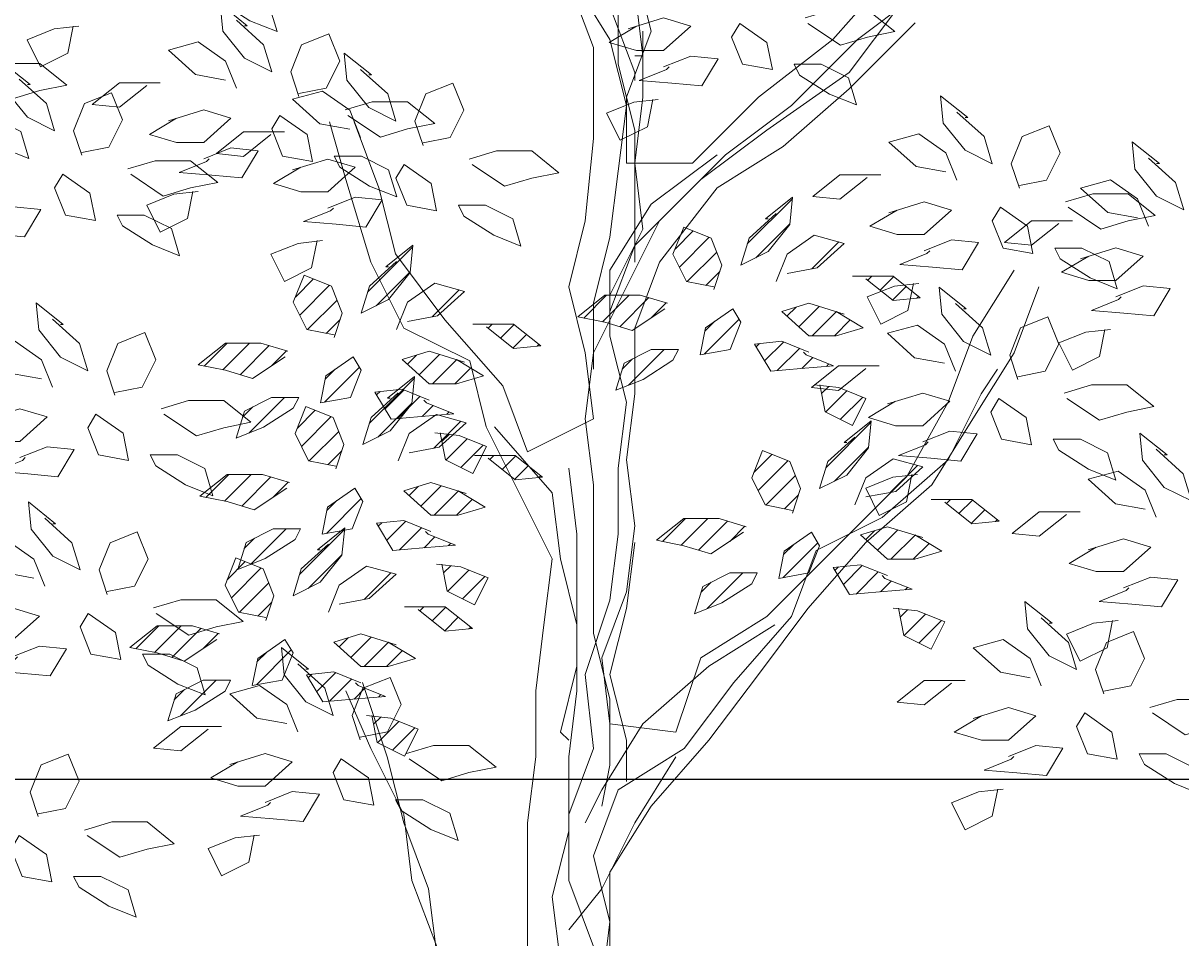
# Model space of a CAD drawing. Units: inches. Extents: x 1770 to 2988, y 1161 to 3221.
# Tile 40 of 44: x 2687 to 2745, y 2750 to 2796. Entities that reach past the tile are written whole.
import ezdxf

# ---------------------------------------------------------------- set-up
doc = ezdxf.new("R2010")
doc.units = ezdxf.units.IN
doc.layers.add('A-ANNO-DIMS', color=2, linetype='Continuous', lineweight=18)
doc.layers.add('trees1', color=250, linetype='Continuous', lineweight=13)
doc.styles.get("Standard").update_dxf_attribs({"font": 'arial.ttf'})
doc.dimstyles.get("Standard").update_dxf_attribs({"dimtxt": 0.18, "dimasz": 0.18, "dimexe": 0.18, "dimexo": 0.0625, "dimgap": 0.09, "dimtad": 0, "dimtih": 1, "dimtoh": 1, "dimdec": 4, "dimzin": 0, "dimdsep": 46, "dimtxsty": 'Standard', "dimcen": 0.09, "dimadec": 0, "dimazin": 0, "dimtfac": 1, "dimtdec": 4, "dimtofl": 0, "dimtmove": 0, "dimatfit": 3, "dimfxl": 1, "dimtolj": 1, "dimtzin": 0, "dimarcsym": 0})

# ---------------------------------------------------------------- blocks, each defined once
blk = doc.blocks.new('*X12')
at = {"color": 0}
for p, q in [((0.47641, -0.84941), (0.49451, -0.83131)), ((0.49114, -0.85236), (0.51219, -0.83131)), ((0.5049, -0.85628), (0.52785, -0.83333)), ((0.52956, -0.8493), (0.54145, -0.83741))]:
    blk.add_line(p, q, dxfattribs=at)
blk = doc.blocks.new('*X10')
at = {"color": 0}
for p, q in [((0.51178, -0.90243), (0.53998, -0.87423)), ((0.50681, -0.88973), (0.5149, -0.88163))]:
    blk.add_line(p, q, dxfattribs=at)
blk = doc.blocks.new('*X15')
at = {"color": 0}
for p, q in [((0.60562, -0.79091), (0.64126, -0.75528)), ((0.61243, -0.80179), (0.63929, -0.77492))]:
    blk.add_line(p, q, dxfattribs=at)
blk = doc.blocks.new('*X14')
at = {"color": 0}
blk.add_line((0.65666, -0.81059), (0.67788, -0.78936), dxfattribs=at)
blk = doc.blocks.new('*X6')
at = {"color": 0}
for p, q in [((0.61933, -0.88328), (0.63423, -0.86837)), ((0.61269, -0.87223), (0.61539, -0.86953)), ((0.62935, -0.89093), (0.64686, -0.87342)), ((0.64878, -0.88917), (0.65735, -0.88061)), ((0.66807, -0.88757), (0.66997, -0.88566))]:
    blk.add_line(p, q, dxfattribs=at)
blk = doc.blocks.new('*X8')
at = {"color": 0}
for p, q in [((0.63698, -0.84795), (0.64414, -0.84079)), ((0.64628, -0.85632), (0.66236, -0.84024)), ((0.65678, -0.8635), (0.67596, -0.84432)), ((0.67446, -0.8635), (0.68701, -0.85095))]:
    blk.add_line(p, q, dxfattribs=at)
blk = doc.blocks.new('*X9')
at = {"color": 0}
for p, q in [((0.70074, -0.81954), (0.70399, -0.81629)), ((0.71057, -0.82739), (0.7213, -0.81666)), ((0.72039, -0.83525), (0.73112, -0.82451)), ((0.73958, -0.83373), (0.74095, -0.83237))]:
    blk.add_line(p, q, dxfattribs=at)
blk = doc.blocks.new('*X7')
at = {"color": 0}
for p, q in [((0.66425, -0.90907), (0.66992, -0.90339)), ((0.66732, -0.92367), (0.68419, -0.9068)), ((0.67911, -0.92956), (0.69682, -0.91184))]:
    blk.add_line(p, q, dxfattribs=at)
blk = doc.blocks.new('*X13')
at = {"color": 0}
for p, q in [((0.54857, -0.79493), (0.56288, -0.78062)), ((0.55195, -0.80923), (0.57551, -0.78567)), ((0.55817, -0.82069), (0.58143, -0.79742)), ((0.5729, -0.82363), (0.58391, -0.81263))]:
    blk.add_line(p, q, dxfattribs=at)
blk = doc.blocks.new('*X11')
at = {"color": 0}
for p, q in [((0.57164, -0.87793), (0.59916, -0.85041)), ((0.57212, -0.85977), (0.57987, -0.85203))]:
    blk.add_line(p, q, dxfattribs=at)
blk = doc.blocks.new('tree342')
at = {"color": 0}
for p, q in [((-39.1, 1419.59), (-39.1, 1315.4)), ((-26.06, 1393.54), (-13.03, 1341.45)), ((130.32, 1334.94), (182.45, 1393.54)), ((-78.19, 1387.03), (-45.61, 1334.94)), ((-58.65, 1328.42), (-78.19, 1380.52)), ((-26.06, 1374.01), (-19.55, 1321.91)), ((202, 1374.01), (149.87, 1334.94)), ((-45.61, 1360.98), (-26.06, 1308.89)), ((182.45, 1360.98), (143.36, 1308.89)), ((195.49, 1347.96), (143.36, 1295.86)), ((-13.03, 1341.45), (-32.58, 1289.35)), ((-19.55, 1289.35), (-19.55, 1341.45)), ((-58.65, 1256.79), (-58.65, 1328.42)), ((-45.61, 1334.94), (-32.58, 1282.84)), ((71.68, 1289.35), (130.32, 1334.94)), ((149.87, 1334.94), (97.74, 1282.84)), ((-19.55, 1321.91), (-26.06, 1321.91)), ((-39.1, 1315.4), (-26.06, 1263.3)), ((-26.06, 1308.89), (-26.06, 1302.38)), ((143.36, 1308.89), (78.19, 1263.3)), ((143.36, 1295.86), (91.23, 1250.28)), ((-32.58, 1282.84), (-39.1, 1230.75)), ((-32.58, 1289.35), (-32.58, 1237.26)), ((-26.06, 1237.26), (-19.55, 1289.35)), ((19.55, 1237.26), (71.68, 1289.35)), ((97.74, 1282.84), (45.61, 1243.77)), ((-254.13, 1224.23), (-267.17, 1269.82)), ((-247.62, 1269.82), (-228.07, 1217.72)), ((-26.06, 1263.3), (-26.06, 1159.11)), ((78.19, 1263.3), (26.06, 1224.23)), ((-65.16, 1191.67), (-58.65, 1256.79)), ((45.61, 1243.77), (-6.52, 1191.67)), ((91.23, 1250.28), (39.1, 1217.72)), ((-32.58, 1237.26), (19.55, 1237.26)), ((-19.55, 1185.16), (-26.06, 1237.26)), ((-39.1, 1230.75), (-45.61, 1178.65)), ((-234.58, 1159.11), (-254.13, 1224.23)), ((-228.07, 1217.72), (-215.04, 1165.63)), ((26.06, 1224.23), (-26.06, 1172.14)), ((39.1, 1217.72), (-6.52, 1159.11)), ((-78.19, 1139.58), (-65.16, 1191.67)), ((-6.52, 1191.67), (-58.65, 1087.48)), ((-45.61, 1133.07), (-19.55, 1185.16)), ((-45.61, 1178.65), (-58.65, 1126.56)), ((-26.06, 1172.14), (-45.61, 1120.04)), ((-215.04, 1165.63), (-175.94, 1113.53)), ((-208.52, 1107.02), (-234.58, 1159.11)), ((-6.52, 1159.11), (-26.06, 1107.02)), ((241.1, 1100.51), (273.68, 1152.6)), ((-65.16, 1087.48), (-78.19, 1139.58)), ((-58.65, 1126.56), (-58.65, 1074.46)), ((-45.61, 1113.53), (-45.61, 1133.07)), ((-45.61, 1120.04), (-45.61, 1113.53)), ((-156.39, 1080.97), (-208.52, 1107.02)), ((-175.94, 1113.53), (-130.32, 1061.44)), ((-26.06, 1107.02), (-26.06, 1054.92)), ((221.55, 1048.41), (241.1, 1100.51)), ((-143.36, 1028.88), (-156.39, 1080.97)), ((-58.65, 1087.48), (-65.16, 1035.39)), ((-58.65, 1035.39), (-65.16, 1087.48)), ((-130.32, 1061.44), (-110.78, 1009.34)), ((-26.06, 1054.92), (-32.58, 1002.83)), ((188.97, 989.81), (221.55, 1048.41)), ((-110.78, 1009.34), (-58.65, 1035.39)), ((-65.16, 1035.39), (-58.65, 983.29)), ((-91.23, 924.69), (-143.36, 1028.88)), ((-32.58, 1002.83), (-26.06, 950.73)), ((-78.19, 996.32), (-71.68, 944.22)), ((78.19, 879.1), (188.97, 989.81)), ((-58.65, 983.29), (-58.65, 866.08)), ((-71.68, 944.22), (-71.68, 840.03)), ((-26.06, 950.73), (-32.58, 898.64)), ((-26.06, 937.71), (-32.58, 885.62)), ((-97.74, 872.59), (-91.23, 924.69)), ((-32.58, 898.64), (-52.13, 846.54)), ((-32.58, 885.62), (-45.61, 833.52)), ((26.06, 846.54), (78.19, 879.1)), ((-104.26, 820.5), (-97.74, 872.59)), ((84.71, 872.59), (32.58, 840.03)), ((-58.65, 866.08), (-45.61, 813.98)), ((-52.13, 846.54), (-45.61, 794.45)), ((6.52, 787.94), (26.06, 846.54)), ((-71.68, 840.03), (-84.71, 787.94)), ((-45.61, 833.52), (-32.58, 781.43)), ((32.58, 840.03), (-19.55, 794.45)), ((-241.1, 827.01), (-221.55, 768.4)), ((-104.26, 768.4), (-104.26, 820.5)), ((-45.61, 813.98), (-45.61, 761.89)), ((-84.71, 787.94), (-78.19, 781.43)), ((-19.55, 794.45), (-52.13, 742.35)), ((-45.61, 794.45), (6.52, 787.94)), ((-32.58, 781.43), (-32.58, 748.87)), ((-221.55, 768.4), (-208.52, 716.31)), ((-110.78, 716.31), (-104.26, 768.4)), ((6.52, 768.4), (-26.06, 716.31)), ((-45.61, 761.89), (-52.13, 729.33)), ((-52.13, 742.35), (-65.16, 716.31)), ((-208.52, 716.31), (-188.97, 664.21)), ((-110.78, 612.12), (-110.78, 716.31)), ((-26.06, 716.31), (-52.13, 664.21)), ((-188.97, 664.21), (-182.45, 612.12)), ((-52.13, 664.21), (-78.19, 631.65))]:
    blk.add_line(p, q, dxfattribs=at)
for points in [[(-336.45, 1373.29), (-314.97, 1362.56), (-308.53, 1341.1), (-330, 1349.68), (-353.63, 1364.71), (-357.92, 1373.29)], [(78.39, 1332.52), (82.69, 1311.06), (59.07, 1315.35), (50.48, 1336.81), (56.92, 1347.54)], [(121.34, 1315.35), (142.82, 1304.62), (149.26, 1283.16), (127.79, 1291.74), (104.16, 1306.77), (99.87, 1315.35)], [(-532.55, 1273), (-511.08, 1262.27), (-504.64, 1240.81), (-526.11, 1249.39), (-549.73, 1264.41), (-554.03, 1273)], [(-284.88, 1259.91), (-280.59, 1238.45), (-304.21, 1242.74), (-312.8, 1264.2), (-306.36, 1274.93)], [(-241.93, 1242.74), (-220.46, 1232.01), (-214.02, 1210.55), (-235.49, 1219.14), (-259.11, 1234.16), (-263.41, 1242.74)], [(-186.8, 1221.09), (-182.51, 1199.63), (-206.13, 1203.92), (-214.72, 1225.38), (-208.28, 1236.11)], [(-456.43, 1213.39), (-452.14, 1191.93), (-475.76, 1196.22), (-484.35, 1217.69), (-477.91, 1228.42)], [(-143.85, 1203.92), (-122.38, 1193.19), (-115.94, 1171.73), (-137.41, 1180.32), (-161.03, 1195.34), (-165.33, 1203.92)], [(284.25, 1187.31), (288.54, 1165.85), (264.92, 1170.14), (256.33, 1191.6), (262.78, 1202.33)], [(-413.48, 1196.22), (-392.01, 1185.49), (-385.57, 1164.03), (-407.04, 1172.62), (-430.66, 1187.64), (-434.96, 1196.22)], [(327.2, 1170.14), (348.67, 1159.41), (355.12, 1137.95), (333.64, 1146.53), (310.02, 1161.55), (305.72, 1170.14)], [(29.91, 1107.26), (25.62, 1085.8), (49.24, 1090.09), (57.83, 1111.55), (51.39, 1122.28)], [(-13.04, 1090.09), (-34.51, 1079.36), (-40.95, 1057.9), (-19.48, 1066.48), (4.14, 1081.5), (8.44, 1090.09)], [(-269.97, 1069.36), (-274.26, 1047.9), (-250.64, 1052.19), (-242.05, 1073.65), (-248.49, 1084.38)], [(-312.92, 1052.19), (-334.39, 1041.46), (-340.83, 1020), (-319.36, 1028.59), (-295.74, 1043.61), (-291.44, 1052.19)], [(283.12, 1036.33), (287.41, 1014.87), (263.79, 1019.16), (255.2, 1040.62), (261.64, 1051.35)], [(-430.19, 1023.94), (-425.9, 1002.48), (-449.52, 1006.78), (-458.11, 1028.24), (-451.67, 1038.97)], [(326.07, 1019.16), (347.54, 1008.43), (353.98, 986.97), (332.51, 995.55), (308.89, 1010.58), (304.59, 1019.16)], [(-387.24, 1006.78), (-365.77, 996.05), (-359.33, 974.59), (-380.8, 983.17), (-404.42, 998.19), (-408.72, 1006.78)], [(-268.62, 965.65), (-272.92, 944.19), (-249.3, 948.48), (-240.71, 969.94), (-247.15, 980.67)], [(-311.57, 948.48), (-333.05, 937.75), (-339.49, 916.29), (-318.02, 924.87), (-294.39, 939.9), (-290.1, 948.48)], [(92.1, 930.79), (87.81, 909.33), (111.43, 913.62), (120.02, 935.08), (113.58, 945.81)], [(49.15, 913.62), (27.68, 902.89), (21.24, 881.43), (42.71, 890.01), (66.33, 905.04), (70.63, 913.62)], [(-436.25, 866.63), (-431.95, 845.17), (-455.57, 849.46), (-464.16, 870.92), (-457.72, 881.65)], [(-323.89, 846.1), (-328.19, 824.64), (-304.57, 828.94), (-295.98, 850.4), (-302.42, 861.13)], [(-393.3, 849.46), (-371.82, 838.73), (-365.38, 817.27), (-386.85, 825.86), (-410.48, 840.88), (-414.77, 849.46)], [(-366.84, 828.94), (-388.32, 818.21), (-394.76, 796.75), (-373.29, 805.33), (-349.66, 820.35), (-345.37, 828.94)], [(350.85, 787.97), (355.15, 766.51), (331.52, 770.81), (322.93, 792.27), (329.38, 803)], [(393.8, 770.81), (415.27, 760.08), (421.72, 738.62), (400.24, 747.2), (376.62, 762.22), (372.32, 770.81)], [(-236.44, 751.67), (-232.15, 730.21), (-255.77, 734.5), (-264.36, 755.96), (-257.92, 766.69)], [(-193.5, 734.5), (-172.02, 723.77), (-165.58, 702.31), (-187.05, 710.9), (-210.67, 725.92), (-214.97, 734.5)], [(-490.74, 691.17), (-486.44, 669.71), (-510.06, 674), (-518.65, 695.46), (-512.21, 706.19)], [(-447.79, 674), (-426.31, 663.27), (-419.87, 641.81), (-441.35, 650.39), (-464.97, 665.41), (-469.26, 674)]]:
    blk.add_lwpolyline(points, close=True, dxfattribs=at)
for points in [[(-340.71, 1350.05), (-319.24, 1330.73), (-312.8, 1309.27), (-334.27, 1320), (-351.45, 1341.46), (-353.6, 1362.92), (-332.12, 1345.75), (-334.27, 1345.75)], [(110.61, 1347.54), (136.38, 1330.37), (157.85, 1336.81), (179.32, 1341.1), (157.85, 1358.27), (129.93, 1358.27), (108.46, 1351.83)], [(-469.59, 1345.39), (-473.88, 1323.93), (-495.36, 1313.2), (-506.09, 1334.66), (-484.62, 1343.25), (-465.29, 1345.39)], [(-31.13, 1343.25), (-3.21, 1351.83), (18.27, 1345.39), (-3.21, 1326.08), (-24.68, 1326.08), (-46.16, 1332.52), (-24.68, 1345.39)], [(-291.32, 1292.1), (-269.85, 1296.39), (-259.11, 1317.86), (-267.7, 1339.32), (-289.18, 1330.73), (-297.77, 1309.27), (-291.32, 1289.96)], [(-340.71, 1296.39), (-349.3, 1317.86), (-370.78, 1332.88), (-394.4, 1326.44), (-372.93, 1307.13), (-349.3, 1302.83)], [(-242.64, 1311.22), (-221.16, 1291.91), (-214.72, 1270.45), (-236.19, 1281.18), (-253.37, 1302.64), (-255.52, 1324.1), (-234.05, 1306.93), (-236.19, 1306.93)], [(-3.21, 1313.2), (18.27, 1321.79), (39.74, 1319.64), (26.86, 1298.18), (3.23, 1300.33), (-22.54, 1302.47), (-1.06, 1311.06), (1.09, 1313.2)], [(-543.29, 1305.19), (-517.52, 1288.02), (-496.05, 1294.46), (-474.57, 1298.75), (-496.05, 1315.92), (-523.96, 1315.92), (-545.44, 1309.48)], [(-512.26, 1303.53), (-490.79, 1284.21), (-484.35, 1262.75), (-505.82, 1273.48), (-523, 1294.94), (-525.15, 1316.4), (-503.67, 1299.23), (-505.82, 1299.23)], [(-411.58, 1298.54), (-433.05, 1281.37), (-454.53, 1283.52), (-433.05, 1300.69), (-400.84, 1300.69)], [(-193.25, 1253.28), (-171.77, 1257.57), (-161.03, 1279.03), (-169.62, 1300.49), (-191.1, 1291.91), (-199.69, 1270.45), (-193.25, 1251.14)], [(-462.87, 1245.58), (-441.4, 1249.88), (-430.66, 1271.34), (-439.25, 1292.8), (-460.73, 1284.21), (-469.32, 1262.75), (-462.87, 1243.44)], [(-242.64, 1257.57), (-251.23, 1279.03), (-272.7, 1294.06), (-296.32, 1287.62), (-274.85, 1268.3), (-251.23, 1264.01)], [(228.42, 1277.44), (249.89, 1258.13), (256.33, 1236.67), (234.86, 1247.4), (217.68, 1268.86), (215.53, 1290.32), (237.01, 1273.15), (234.86, 1273.15)], [(-252.67, 1274.93), (-226.9, 1257.77), (-205.43, 1264.2), (-183.95, 1268.5), (-205.43, 1285.66), (-233.34, 1285.66), (-254.82, 1279.23)], [(-11.8, 1287.45), (-16.09, 1265.99), (-37.57, 1255.26), (-48.31, 1276.72), (-26.83, 1285.31), (-7.5, 1287.45)], [(-394.4, 1270.64), (-366.48, 1279.23), (-345.01, 1272.79), (-366.48, 1253.47), (-387.96, 1253.47), (-409.43, 1259.91), (-387.96, 1272.79)], [(277.81, 1219.5), (299.28, 1223.79), (310.02, 1245.25), (301.43, 1266.71), (279.95, 1258.13), (271.37, 1236.67), (277.81, 1217.35)], [(-313.5, 1259.72), (-334.98, 1242.55), (-356.45, 1244.7), (-334.98, 1261.87), (-302.77, 1261.87)], [(228.42, 1223.79), (219.83, 1245.25), (198.35, 1260.27), (174.73, 1253.83), (196.2, 1234.52), (219.83, 1230.23)], [(379.78, 1241.14), (401.26, 1221.82), (407.7, 1200.36), (386.22, 1211.09), (369.04, 1232.55), (366.9, 1254.01), (388.37, 1236.84), (386.22, 1236.84)], [(-366.48, 1240.6), (-345.01, 1249.18), (-323.53, 1247.04), (-336.42, 1225.58), (-360.04, 1227.72), (-385.81, 1229.87), (-364.34, 1238.45), (-362.19, 1240.6)], [(-154.59, 1236.11), (-128.82, 1218.95), (-107.35, 1225.38), (-85.87, 1229.68), (-107.35, 1246.84), (-135.27, 1246.84), (-156.74, 1240.41)], [(39.1, 1243.77), (-13.03, 1204.7), (-45.61, 1152.6), (-45.61, 1100.51), (-32.58, 1048.41), (-39.1, 996.32), (-39.1, 944.22), (-45.61, 892.13), (-65.16, 833.52), (-58.65, 774.91), (-78.19, 722.82), (-78.19, 670.72), (-58.65, 618.63), (-65.16, 566.53), (-65.16, 514.44), (-78.19, 462.34), (-84.71, 410.25), (-84.71, 306.06), (-78.19, 247.45), (-71.68, 195.36), (-78.19, 143.26), (-71.68, 91.17), (-65.16, 32.56), (-65.16, 0)], [(-424.22, 1228.42), (-398.45, 1211.25), (-376.98, 1217.69), (-355.5, 1221.98), (-376.98, 1239.15), (-404.89, 1239.15), (-426.37, 1232.71)], [(-296.32, 1231.82), (-268.41, 1240.41), (-246.93, 1233.97), (-268.41, 1214.65), (-289.88, 1214.65), (-311.36, 1221.09), (-289.88, 1233.97)], [(157.55, 1225.94), (136.08, 1208.77), (114.6, 1210.91), (136.08, 1228.08), (168.29, 1228.08)], [(379.78, 1187.49), (371.19, 1208.95), (349.72, 1223.97), (326.09, 1217.53), (347.57, 1198.22), (371.19, 1193.92)], [(-375.07, 1214.85), (-379.37, 1193.39), (-400.84, 1182.66), (-411.58, 1204.12), (-390.11, 1212.7), (-370.78, 1214.85)], [(-268.41, 1201.78), (-246.93, 1210.36), (-225.46, 1208.22), (-238.34, 1186.76), (-261.96, 1188.9), (-287.73, 1191.05), (-266.26, 1199.63), (-264.11, 1201.78)], [(85.75, 1197.39), (64.27, 1178.07), (57.83, 1156.61), (79.3, 1167.34), (96.48, 1188.8), (98.63, 1210.26), (77.16, 1193.1), (79.3, 1193.1)], [(316.46, 1202.33), (342.23, 1185.16), (363.71, 1191.6), (385.18, 1195.89), (363.71, 1213.06), (335.79, 1213.06), (314.31, 1206.62)], [(-538.03, 1194.08), (-516.56, 1202.66), (-495.09, 1200.52), (-507.97, 1179.06), (-531.59, 1181.2), (-557.36, 1183.35), (-535.89, 1191.93), (-533.74, 1194.08)], [(174.73, 1198.04), (202.65, 1206.62), (224.12, 1200.18), (202.65, 1180.87), (181.17, 1180.87), (159.7, 1187.31), (181.17, 1200.18)], [(308.92, 1189.63), (287.44, 1172.46), (265.97, 1174.61), (287.44, 1191.78), (319.65, 1191.78)], [(36.36, 1139.45), (14.88, 1143.74), (4.14, 1165.2), (12.73, 1186.66), (34.21, 1178.07), (42.8, 1156.61), (36.36, 1137.3)], [(85.75, 1143.74), (94.34, 1165.2), (115.81, 1180.22), (139.43, 1173.78), (117.96, 1154.47), (94.34, 1150.18)], [(-277, 1176.03), (-281.29, 1154.57), (-302.77, 1143.84), (-313.5, 1165.3), (-292.03, 1173.88), (-272.7, 1176.03)], [(-214.14, 1159.49), (-235.61, 1140.18), (-242.05, 1118.72), (-220.58, 1129.45), (-203.4, 1150.91), (-201.25, 1172.37), (-222.72, 1155.2), (-220.58, 1155.2)], [(202.65, 1167.99), (224.12, 1176.58), (245.6, 1174.43), (232.71, 1152.97), (209.09, 1155.12), (183.32, 1157.26), (204.79, 1165.85), (206.94, 1167.99)], [(326.09, 1161.73), (354.01, 1170.32), (375.49, 1163.88), (354.01, 1144.57), (332.54, 1144.57), (311.06, 1151), (332.54, 1163.88)], [(-263.53, 1101.55), (-285, 1105.84), (-295.74, 1127.3), (-287.15, 1148.76), (-265.67, 1140.18), (-257.08, 1118.72), (-263.53, 1099.4)], [(156.61, 1145.88), (178.09, 1128.72), (199.56, 1130.86), (178.09, 1148.03), (145.88, 1148.03)], [(-214.14, 1105.84), (-205.55, 1127.3), (-184.07, 1142.32), (-160.45, 1135.89), (-181.92, 1116.57), (-205.55, 1112.28)], [(293.23, 1139.58), (273.68, 1087.48), (241.1, 1035.39), (208.52, 983.29), (156.39, 937.71), (110.78, 885.62), (71.68, 833.52), (32.58, 781.43), (-13.03, 729.33), (-45.61, 677.24), (-45.61, 566.53), (-39.1, 507.93), (-45.61, 455.83), (-45.61, 403.74), (-39.1, 345.13), (-58.65, 293.03), (-58.65, 188.84), (-65.16, 136.75), (-58.65, 84.65), (-52.13, 32.56), (-45.61, 13.02)], [(194.06, 1142.24), (189.76, 1120.78), (168.29, 1110.05), (157.55, 1131.51), (179.03, 1140.09), (198.35, 1142.24)], [(227.28, 1126.46), (248.76, 1107.15), (255.2, 1085.69), (233.73, 1096.42), (216.55, 1117.88), (214.4, 1139.34), (235.87, 1122.17), (233.73, 1122.17)], [(354.01, 1131.69), (375.49, 1140.27), (396.96, 1138.13), (384.08, 1116.67), (360.45, 1118.81), (334.68, 1120.96), (356.16, 1129.54), (358.31, 1131.69)], [(-486.02, 1114.08), (-464.55, 1094.76), (-458.11, 1073.3), (-479.58, 1084.03), (-496.76, 1105.49), (-498.91, 1126.95), (-477.43, 1109.78), (-479.58, 1109.78)], [(-2.3, 1122.28), (-28.07, 1105.11), (-49.54, 1111.55), (-71.02, 1115.84), (-49.54, 1133.01), (-21.63, 1133.01), (-0.15, 1126.57)], [(139.43, 1117.99), (111.52, 1126.57), (90.04, 1120.13), (111.52, 1100.82), (132.99, 1100.82), (154.46, 1107.26), (132.99, 1120.13)], [(276.68, 1068.52), (298.15, 1072.81), (308.89, 1094.27), (300.3, 1115.73), (278.82, 1107.15), (270.23, 1085.69), (276.68, 1066.37)], [(-143.27, 1107.99), (-121.8, 1090.82), (-100.32, 1092.97), (-121.8, 1110.13), (-154.01, 1110.13)], [(227.28, 1072.81), (218.69, 1094.27), (197.22, 1109.29), (173.6, 1102.85), (195.07, 1083.54), (218.69, 1079.25)], [(-436.63, 1056.13), (-415.16, 1060.43), (-404.42, 1081.89), (-413.01, 1103.35), (-434.49, 1094.76), (-443.08, 1073.3), (-436.63, 1053.99)], [(345.42, 1105.94), (341.13, 1084.48), (319.65, 1073.75), (308.92, 1095.21), (330.39, 1103.79), (349.72, 1105.94)], [(-486.02, 1060.43), (-494.61, 1081.89), (-516.09, 1096.91), (-539.71, 1090.47), (-518.24, 1071.16), (-494.61, 1066.86)], [(-302.18, 1084.38), (-327.95, 1067.21), (-349.42, 1073.65), (-370.9, 1077.94), (-349.42, 1095.11), (-321.51, 1095.11), (-300.03, 1088.67)], [(-160.45, 1080.09), (-188.37, 1088.67), (-209.84, 1082.24), (-188.37, 1062.92), (-166.89, 1062.92), (-145.42, 1069.36), (-166.89, 1082.24)], [(111.52, 1087.94), (90.04, 1096.53), (68.57, 1094.38), (81.45, 1072.92), (105.07, 1075.07), (130.84, 1077.21), (109.37, 1085.8), (107.22, 1087.94)], [(-65.16, 6.51), (-91.23, 58.61), (-84.71, 110.7), (-84.71, 162.8), (-78.19, 214.89), (-58.65, 266.99), (-52.13, 319.08), (-65.16, 371.18), (-52.13, 429.78), (-52.13, 481.88), (-45.61, 533.97), (-52.13, 586.07), (-45.61, 638.16), (-58.65, 690.26), (-39.1, 742.35), (13.03, 774.91), (52.13, 827.01), (97.74, 879.1), (117.29, 931.2), (169.42, 957.25), (221.55, 1002.83), (247.62, 1054.92), (260.65, 1074.46)], [(156.42, 1074.96), (134.94, 1057.79), (113.47, 1059.93), (134.94, 1077.1), (167.16, 1077.1)], [(-212.79, 1055.78), (-234.27, 1036.47), (-240.71, 1015.01), (-219.23, 1025.74), (-202.05, 1047.2), (-199.91, 1068.66), (-221.38, 1051.49), (-219.23, 1051.49)], [(120.11, 1062.19), (124.4, 1040.73), (145.88, 1030), (156.61, 1051.46), (135.14, 1060.04), (115.81, 1062.19)], [(315.33, 1051.35), (341.1, 1034.18), (362.57, 1040.62), (384.05, 1044.91), (362.57, 1062.08), (334.66, 1062.08), (313.18, 1055.64)], [(-188.37, 1050.05), (-209.84, 1058.63), (-231.31, 1056.48), (-218.43, 1035.02), (-194.81, 1037.17), (-169.04, 1039.32), (-190.51, 1047.9), (-192.66, 1050.05)], [(173.6, 1047.06), (201.52, 1055.64), (222.99, 1049.2), (201.52, 1029.89), (180.04, 1029.89), (158.57, 1036.33), (180.04, 1049.2)], [(-539.71, 1034.67), (-511.79, 1043.26), (-490.32, 1036.82), (-511.79, 1017.51), (-533.27, 1017.51), (-554.74, 1023.94), (-533.27, 1036.82)], [(-397.98, 1038.97), (-372.21, 1021.8), (-350.74, 1028.24), (-329.26, 1032.53), (-350.74, 1049.7), (-378.65, 1049.7), (-400.13, 1043.26)], [(-262.18, 997.84), (-283.66, 1002.13), (-294.39, 1023.59), (-285.8, 1045.05), (-264.33, 1036.47), (-255.74, 1015.01), (-262.18, 995.69)], [(-212.79, 1002.13), (-204.2, 1023.59), (-182.73, 1038.61), (-159.11, 1032.17), (-180.58, 1012.86), (-204.2, 1008.57)], [(147.94, 1020.92), (126.46, 1001.61), (120.02, 980.15), (141.49, 990.88), (158.67, 1012.34), (160.82, 1033.8), (139.35, 1016.63), (141.49, 1016.63)], [(-179.78, 1024.29), (-175.48, 1002.83), (-154.01, 992.1), (-143.27, 1013.56), (-164.74, 1022.15), (-184.07, 1024.29)], [(-136.84, 1028.88), (-91.23, 976.78), (-84.71, 924.69), (-71.68, 872.59), (-71.68, 820.5), (-78.19, 768.4), (-78.19, 709.79), (-91.23, 657.7), (-84.71, 605.6), (-78.19, 553.51), (-84.71, 501.41), (-97.74, 449.32), (-97.74, 410.25)], [(201.52, 1017.01), (222.99, 1025.6), (244.46, 1023.45), (231.58, 1001.99), (207.96, 1004.14), (182.19, 1006.28), (203.66, 1014.87), (205.81, 1017.01)], [(385.84, 1011.22), (407.31, 991.9), (413.75, 970.44), (392.28, 981.17), (375.1, 1002.63), (372.95, 1024.09), (394.43, 1006.93), (392.28, 1006.93)], [(-511.79, 1004.63), (-490.32, 1013.21), (-468.84, 1011.07), (-481.73, 989.61), (-505.35, 991.75), (-531.12, 993.9), (-509.65, 1002.48), (-507.5, 1004.63)], [(-141.93, 1004.28), (-120.45, 987.11), (-98.98, 989.25), (-120.45, 1006.42), (-152.66, 1006.42)], [(98.54, 962.98), (77.07, 967.27), (66.33, 988.73), (74.92, 1010.19), (96.4, 1001.61), (104.99, 980.15), (98.54, 960.83)], [(147.94, 967.27), (156.53, 988.73), (178, 1003.75), (201.62, 997.31), (180.15, 978), (156.53, 973.71)], [(-300.84, 980.67), (-326.61, 963.5), (-348.08, 969.94), (-369.55, 974.23), (-348.08, 991.4), (-320.16, 991.4), (-298.69, 984.96)], [(192.93, 991.26), (188.63, 969.8), (167.16, 959.07), (156.42, 980.53), (177.89, 989.12), (197.22, 991.26)], [(385.84, 957.57), (377.25, 979.03), (355.77, 994.05), (332.15, 987.61), (353.62, 968.3), (377.25, 964.01)], [(-159.11, 976.38), (-187.02, 984.96), (-208.5, 978.52), (-187.02, 959.21), (-165.55, 959.21), (-144.07, 965.65), (-165.55, 978.52)], [(-492.08, 956.76), (-470.6, 937.45), (-464.16, 915.99), (-485.64, 926.72), (-502.82, 948.18), (-504.96, 969.64), (-483.49, 952.47), (-485.64, 952.47)], [(218.8, 969.42), (240.28, 952.25), (261.75, 954.39), (240.28, 971.56), (208.06, 971.56)], [(314.97, 959.71), (293.5, 942.54), (272.02, 944.69), (293.5, 961.86), (325.71, 961.86)], [(-187.02, 946.33), (-208.5, 954.92), (-229.97, 952.77), (-217.09, 931.31), (-193.46, 933.46), (-167.69, 935.6), (-189.17, 944.19), (-191.32, 946.33)], [(59.89, 945.81), (34.12, 928.64), (12.65, 935.08), (-8.83, 939.37), (12.65, 956.54), (40.56, 956.54), (62.04, 950.1)], [(-442.69, 898.82), (-421.21, 903.11), (-410.48, 924.57), (-419.07, 946.03), (-440.54, 937.45), (-449.13, 915.99), (-442.69, 896.67)], [(-268.06, 936.24), (-289.54, 916.92), (-295.98, 895.46), (-274.5, 906.19), (-257.32, 927.65), (-255.18, 949.11), (-276.65, 931.94), (-274.5, 931.94)], [(201.62, 941.52), (173.71, 950.1), (152.23, 943.66), (173.71, 924.35), (195.18, 924.35), (216.65, 930.79), (195.18, 943.66)], [(-492.08, 903.11), (-500.67, 924.57), (-522.14, 939.59), (-545.77, 933.16), (-524.29, 913.84), (-500.67, 909.55)], [(332.15, 931.81), (360.07, 940.4), (381.54, 933.96), (360.07, 914.65), (338.59, 914.65), (317.12, 921.08), (338.59, 933.96)], [(-317.45, 878.29), (-338.93, 882.59), (-349.66, 904.05), (-341.07, 925.51), (-319.6, 916.92), (-311.01, 895.46), (-317.45, 876.15)], [(-268.06, 882.59), (-259.47, 904.05), (-238, 919.07), (-214.37, 912.63), (-235.85, 893.32), (-259.47, 889.02)], [(-178.43, 920.58), (-174.14, 899.12), (-152.66, 888.39), (-141.93, 909.85), (-163.4, 918.44), (-182.73, 920.58)], [(173.71, 911.47), (152.23, 920.06), (130.76, 917.91), (143.64, 896.45), (167.26, 898.6), (193.03, 900.74), (171.56, 909.33), (169.41, 911.47)], [(360.07, 901.77), (381.54, 910.35), (403.01, 908.21), (390.13, 886.75), (366.51, 888.89), (340.74, 891.04), (362.21, 899.62), (364.36, 901.77)], [(-404.03, 881.65), (-378.26, 864.48), (-356.79, 870.92), (-335.32, 875.21), (-356.79, 892.38), (-384.71, 892.38), (-406.18, 885.94)], [(295.02, 878.11), (316.49, 858.79), (322.93, 837.33), (301.46, 848.06), (284.28, 869.52), (282.13, 890.98), (303.61, 873.81), (301.46, 873.81)], [(-545.77, 877.36), (-517.85, 885.94), (-496.37, 879.51), (-517.85, 860.19), (-539.32, 860.19), (-560.8, 866.63), (-539.32, 879.51)], [(-197.2, 884.73), (-175.72, 867.56), (-154.25, 869.71), (-175.72, 886.88), (-207.93, 886.88)], [(182.29, 885.72), (186.59, 864.26), (208.06, 853.53), (218.8, 874.99), (197.33, 883.58), (178, 885.72)], [(-356.11, 861.13), (-381.88, 843.96), (-403.35, 850.4), (-424.82, 854.69), (-403.35, 871.86), (-375.43, 871.86), (-353.96, 865.42)], [(351.48, 876.02), (347.18, 854.56), (325.71, 843.83), (314.97, 865.29), (336.44, 873.87), (355.77, 876.02)], [(-214.37, 856.83), (-242.29, 865.42), (-263.77, 858.98), (-242.29, 839.67), (-220.82, 839.67), (-199.34, 846.1), (-220.82, 858.98)], [(295.02, 824.46), (286.43, 845.92), (264.95, 860.94), (241.33, 854.5), (262.8, 835.19), (286.43, 830.89)], [(344.41, 820.16), (365.88, 824.46), (376.62, 845.92), (368.03, 867.38), (346.56, 858.79), (337.97, 837.33), (344.41, 818.02)], [(-517.85, 847.32), (-496.37, 855.9), (-474.9, 853.75), (-487.78, 832.29), (-511.41, 834.44), (-537.18, 836.59), (-515.7, 845.17), (-513.55, 847.32)], [(-292.28, 841.8), (-270.8, 822.49), (-264.36, 801.03), (-285.84, 811.76), (-303.02, 833.22), (-305.16, 854.68), (-283.69, 837.51), (-285.84, 837.51)], [(-242.29, 826.79), (-263.77, 835.37), (-285.24, 833.23), (-272.36, 811.77), (-248.73, 813.91), (-222.96, 816.06), (-244.44, 824.64), (-246.59, 826.79)], [(-292.28, 788.15), (-300.87, 809.61), (-322.34, 824.64), (-345.96, 818.2), (-324.49, 798.88), (-300.87, 794.59)], [(-242.89, 783.86), (-221.41, 788.15), (-210.67, 809.61), (-219.26, 831.07), (-240.74, 822.49), (-249.33, 801.03), (-242.89, 781.72)], [(224.15, 826.6), (202.68, 809.43), (181.2, 811.58), (202.68, 828.75), (234.89, 828.75)], [(-162.91, 26.05), (-149.87, 78.14), (-143.36, 130.24), (-136.84, 188.84), (-130.32, 240.94), (-123.81, 293.03), (-110.78, 351.64), (-117.29, 403.74), (-136.84, 455.83), (-156.39, 514.44), (-175.94, 566.53), (-182.45, 618.63), (-202, 670.72), (-208.52, 722.82), (-234.58, 774.91), (-254.13, 820.5)], [(241.33, 798.7), (269.25, 807.29), (290.72, 800.85), (269.25, 781.54), (247.77, 781.54), (226.3, 787.97), (247.77, 800.85)], [(383.06, 803), (408.83, 785.83), (430.31, 792.27), (451.78, 796.56), (430.31, 813.73), (402.39, 813.73), (380.91, 807.29)], [(-233.7, 801.04), (-229.41, 779.58), (-207.93, 768.85), (-197.2, 790.31), (-218.67, 798.89), (-238, 801.04)], [(-363.14, 790.3), (-384.62, 773.13), (-406.09, 775.28), (-384.62, 792.45), (-352.41, 792.45)], [(-204.23, 766.69), (-178.46, 749.52), (-156.99, 755.96), (-135.51, 760.26), (-156.99, 777.42), (-184.91, 777.42), (-206.38, 770.99)], [(-497.18, 723.36), (-475.7, 727.65), (-464.97, 749.11), (-473.56, 770.57), (-495.03, 761.98), (-503.62, 740.52), (-497.18, 721.21)], [(-345.96, 762.4), (-318.05, 770.99), (-296.57, 764.55), (-318.05, 745.23), (-339.52, 745.23), (-361, 751.67), (-339.52, 764.55)], [(269.25, 768.66), (290.72, 777.24), (312.2, 775.1), (299.31, 753.64), (275.69, 755.78), (249.92, 757.93), (271.39, 766.51), (273.54, 768.66)], [(-318.05, 732.36), (-296.57, 740.94), (-275.1, 738.79), (-287.98, 717.33), (-311.6, 719.48), (-337.37, 721.63), (-315.9, 730.21), (-313.75, 732.36)], [(260.66, 742.91), (256.36, 721.45), (234.89, 710.72), (224.15, 732.18), (245.63, 740.76), (264.95, 742.91)], [(-458.53, 706.19), (-432.76, 689.02), (-411.28, 695.46), (-389.81, 699.75), (-411.28, 716.92), (-439.2, 716.92), (-460.67, 710.48)], [(-326.64, 706.6), (-330.93, 685.14), (-352.41, 674.41), (-363.14, 695.87), (-341.67, 704.46), (-322.34, 706.6)]]:
    blk.add_lwpolyline(points, dxfattribs=at)
at = {"color": 0, "xscale": 1000, "yscale": 1000, "zscale": 1000}
for name, p in [('*X15', (-542.75, 1964.32)), ('*X13', (-542.75, 1964.32)), ('*X15', (-842.63, 1926.42)), ('*X14', (-542.75, 1964.32)), ('*X13', (-842.63, 1926.42)), ('*X9', (-542.75, 1964.32)), ('*X14', (-842.63, 1926.42)), ('*X12', (-542.75, 1964.32)), ('*X8', (-542.75, 1964.32)), ('*X9', (-842.63, 1926.42)), ('*X11', (-542.75, 1964.32)), ('*X12', (-842.63, 1926.42)), ('*X10', (-542.75, 1964.32)), ('*X6', (-542.75, 1964.32)), ('*X8', (-842.63, 1926.42)), ('*X11', (-842.63, 1926.42)), ('*X15', (-841.29, 1822.71)), ('*X7', (-542.75, 1964.32)), ('*X10', (-842.63, 1926.42)), ('*X6', (-842.63, 1926.42)), ('*X13', (-841.29, 1822.71)), ('*X14', (-841.29, 1822.71)), ('*X15', (-480.56, 1787.85)), ('*X7', (-842.63, 1926.42)), ('*X9', (-841.29, 1822.71)), ('*X13', (-480.56, 1787.85)), ('*X14', (-480.56, 1787.85)), ('*X12', (-841.29, 1822.71)), ('*X8', (-841.29, 1822.71)), ('*X11', (-841.29, 1822.71)), ('*X9', (-480.56, 1787.85)), ('*X6', (-841.29, 1822.71)), ('*X12', (-480.56, 1787.85)), ('*X10', (-841.29, 1822.71)), ('*X15', (-896.56, 1703.17)), ('*X8', (-480.56, 1787.85)), ('*X11', (-480.56, 1787.85)), ('*X13', (-896.56, 1703.17)), ('*X7', (-841.29, 1822.71)), ('*X6', (-480.56, 1787.85)), ('*X14', (-896.56, 1703.17)), ('*X10', (-480.56, 1787.85)), ('*X9', (-896.56, 1703.17)), ('*X7', (-480.56, 1787.85)), ('*X12', (-896.56, 1703.17)), ('*X8', (-896.56, 1703.17)), ('*X11', (-896.56, 1703.17)), ('*X6', (-896.56, 1703.17)), ('*X10', (-896.56, 1703.17)), ('*X7', (-896.56, 1703.17))]:
    blk.add_blockref(name, p, dxfattribs=at)
blk = doc.blocks.new('*D96')
at = {"layer": 'A-ANNO-DIMS', "color": 0, "lineweight": -2, "transparency": 16777216}
for p, q in [((2620.113, 2758.297), (2801.915, 2758.297)), ((2801.735, 2758.117), (2801.735, 2740.479)), ((2801.735, 2722.477), (2801.735, 2740.115)), ((2655.505, 2722.297), (2801.915, 2722.297))]:
    blk.add_line(p, q, dxfattribs=at)
at = {"layer": 'A-ANNO-DIMS', "color": 0, "transparency": 16777216}
for points in [[(2801.705, 2758.117), (2801.765, 2758.117), (2801.735, 2758.297)], [(2801.705, 2722.477), (2801.765, 2722.477), (2801.735, 2722.297)]]:
    blk.add_solid(points, dxfattribs=at)
at = {"layer": 'Defpoints', "color": 0, "transparency": 16777216}
for p in [(2620.051, 2758.297), (2801.735, 2758.297), (2655.443, 2722.297)]:
    blk.add_point(p, dxfattribs=at)
at = {"layer": 'A-ANNO-DIMS', "color": 0, "transparency": 16777216, "insert": (2801.735, 2740.297), "char_height": 0.18, "attachment_point": 5}
blk.add_mtext('\\A1;36', dxfattribs=at)
blk = doc.blocks.new('*D97')
at = {"layer": 'A-ANNO-DIMS', "color": 0, "lineweight": -2, "transparency": 16777216}
for p, q in [((2620.113, 2806.297), (2801.915, 2806.297)), ((2801.735, 2806.117), (2801.735, 2782.479)), ((2801.735, 2758.477), (2801.735, 2782.115)), ((2620.113, 2758.297), (2801.915, 2758.297))]:
    blk.add_line(p, q, dxfattribs=at)
at = {"layer": 'A-ANNO-DIMS', "color": 0, "transparency": 16777216}
for points in [[(2801.705, 2806.117), (2801.765, 2806.117), (2801.735, 2806.297)], [(2801.705, 2758.477), (2801.765, 2758.477), (2801.735, 2758.297)]]:
    blk.add_solid(points, dxfattribs=at)
at = {"layer": 'Defpoints', "color": 0, "transparency": 16777216}
for p in [(2620.051, 2806.297), (2801.735, 2806.297), (2620.051, 2758.297)]:
    blk.add_point(p, dxfattribs=at)
at = {"layer": 'A-ANNO-DIMS', "color": 0, "transparency": 16777216, "insert": (2801.735, 2782.297), "char_height": 0.18, "attachment_point": 5}
blk.add_mtext('\\A1;48', dxfattribs=at)

msp = doc.modelspace()

# ---------------------------------------------------------------- block references
at = {"layer": 'trees1', "xscale": 0.063143750371755, "yscale": 0.063143750371755, "zscale": 0.063143750371755}
msp.add_blockref('tree342', (2719.3275, 2710.8976), dxfattribs=at)

# ---------------------------------------------------------------- dimensions: what is measured, and where the dimension line sits
at = {"layer": 'A-ANNO-DIMS'}
for base, p1, p2, picture, middle in [((2801.7346, 2806.2969), (2620.0508, 2758.2969), (2620.0508, 2806.2969), '*D97', (2801.7346, 2782.2969)), ((2801.7346, 2758.2969), (2655.443, 2722.2969), (2620.0508, 2758.2969), '*D96', (2801.7346, 2740.2969))]:
    dim = msp.add_linear_dim(base=base, p1=p1, p2=p2, angle=90, dimstyle='Standard', override={"dimdec": 0, "dimlfac": 1, "dimrnd": 0, "dimzin": 0, "dimdsep": 46, "dimlunit": 2}, dxfattribs=at)
    dim.commit()
    dim.dimension.update_dxf_attribs({"geometry": picture, "text_midpoint": middle})

doc.saveas('drawing.dxf')
